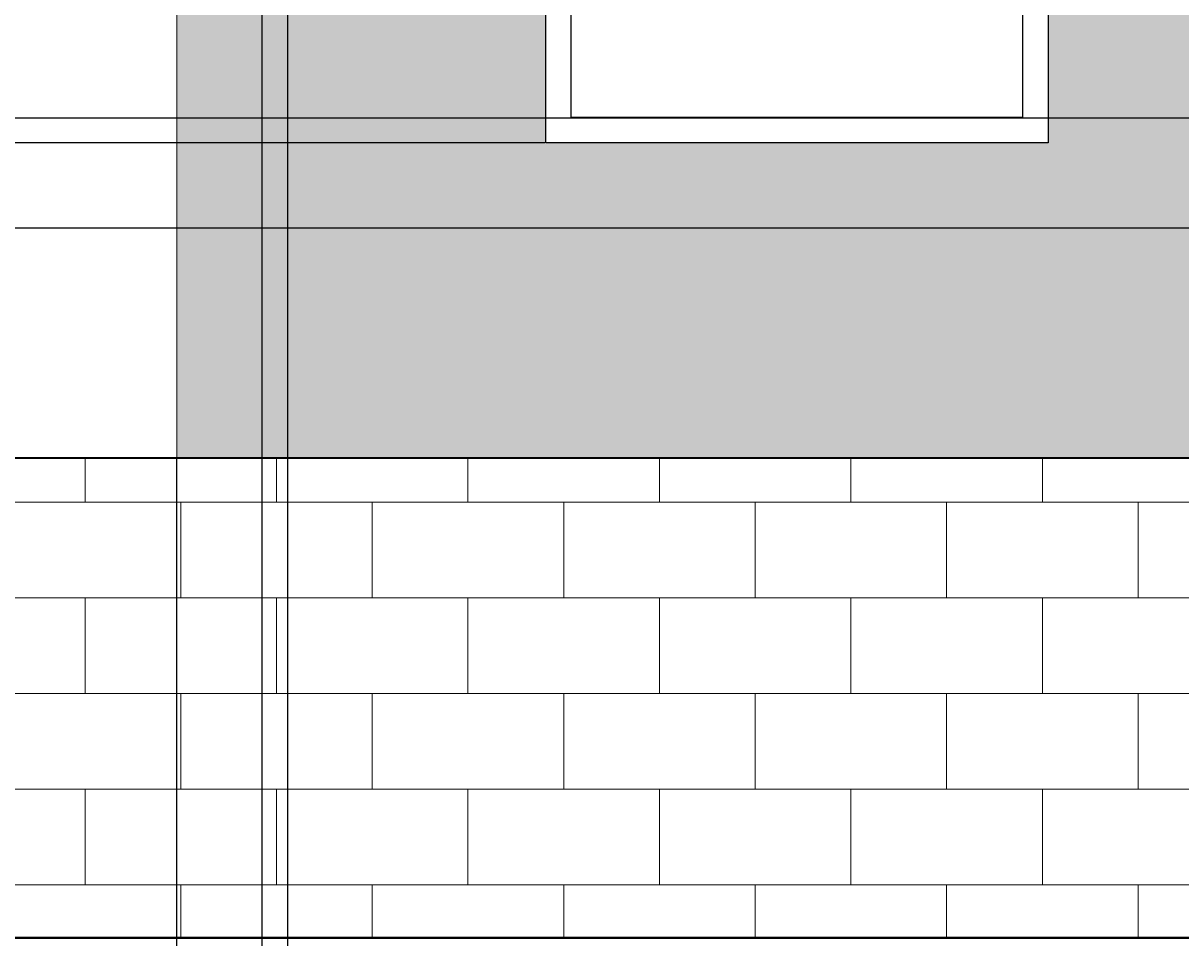
# Model space of a CAD drawing. Units: inches. Extents: x -13 to 809, y 112 to 656.
# Tile 23 of 55: x 430 to 521, y 251 to 323. Entities that reach past the tile are written whole.
import ezdxf

# ---------------------------------------------------------------- set-up
doc = ezdxf.new("R2010")
doc.units = ezdxf.units.IN
doc.header["$MEASUREMENT"] = 0
for name, color, linetype, lineweight in [('A-ANNO-DIMS', 2, 'Continuous', 18), ('A-ELEV', 7, 'Continuous', 35), ('A-ELEV-PATT', 8, 'Continuous', 13), ('A-GLAZ', 4, 'Continuous', 25)]:
    doc.layers.add(name, color=color, linetype=linetype, lineweight=lineweight)
doc.styles.get("Standard").update_dxf_attribs({"font": 'arial.ttf'})
doc.dimstyles.get("Standard").update_dxf_attribs({"dimtxt": 0.625, "dimasz": 0.18, "dimexe": 0.18, "dimexo": 0.0625, "dimgap": 0.09, "dimtad": 0, "dimtih": 1, "dimtoh": 1, "dimdec": 4, "dimzin": 0, "dimdsep": 46, "dimlunit": 4, "dimtxsty": 'Standard', "dimcen": 0.09, "dimadec": 0, "dimazin": 0, "dimtfac": 1, "dimtdec": 4, "dimtofl": 0, "dimtmove": 0, "dimatfit": 3, "dimfxl": 1, "dimtolj": 1, "dimtzin": 0, "dimarcsym": 0})

# ---------------------------------------------------------------- blocks, each defined once
blk = doc.blocks.new('WIN-FIXED-400')
for points in [[(0, 27.268), (39.362, 27.268), (39.362, 0), (0, 0)], [(2, 25.268), (37.362, 25.268), (37.362, 2), (2, 2)]]:
    blk.add_lwpolyline(points, close=True)
blk = doc.blocks.new('*D40')
at = {"layer": 'A-ANNO-DIMS', "color": 0, "lineweight": -2, "transparency": 16777216}
for p, q in [((471.037, 313.167), (-12.099, 313.167)), ((-11.919, 312.987), (-11.919, 301.218)), ((-11.919, 288.631), (-11.919, 300.4)), ((341.345, 288.451), (-12.099, 288.451))]:
    blk.add_line(p, q, dxfattribs=at)
at = {"layer": 'A-ANNO-DIMS', "color": 0, "transparency": 16777216}
for points in [[(-11.949, 312.987), (-11.889, 312.987), (-11.919, 313.167)], [(-11.949, 288.631), (-11.889, 288.631), (-11.919, 288.451)]]:
    blk.add_solid(points, dxfattribs=at)
at = {"layer": 'Defpoints', "color": 0, "transparency": 16777216}
for p in [(471.1, 313.167), (-11.919, 288.451), (341.407, 288.451)]:
    blk.add_point(p, dxfattribs=at)
at = {"layer": 'A-ANNO-DIMS', "color": 0, "transparency": 16777216, "insert": (-11.919, 300.809), "char_height": 0.625, "attachment_point": 5}
blk.add_mtext('\\A1;24.716', dxfattribs=at)
blk = doc.blocks.new('*D41')
at = {"layer": 'A-ANNO-DIMS', "color": 0, "lineweight": -2, "transparency": 16777216}
for p, q in [((471.037, 357.98), (-12.099, 357.98)), ((-11.919, 357.8), (-11.919, 335.983)), ((-11.919, 313.347), (-11.919, 335.164)), ((471.037, 313.167), (-12.099, 313.167))]:
    blk.add_line(p, q, dxfattribs=at)
at = {"layer": 'A-ANNO-DIMS', "color": 0, "transparency": 16777216}
for points in [[(-11.949, 357.8), (-11.889, 357.8), (-11.919, 357.98)], [(-11.949, 313.347), (-11.889, 313.347), (-11.919, 313.167)]]:
    blk.add_solid(points, dxfattribs=at)
at = {"layer": 'Defpoints', "color": 0, "transparency": 16777216}
for p in [(-11.919, 357.98), (471.1, 357.98), (471.1, 313.167)]:
    blk.add_point(p, dxfattribs=at)
at = {"layer": 'A-ANNO-DIMS', "color": 0, "transparency": 16777216, "insert": (-11.919, 335.574), "char_height": 0.625, "attachment_point": 5}
blk.add_mtext('\\A1;44.81', dxfattribs=at)
blk = doc.blocks.new('*D51')
at = {"layer": 'A-ANNO-DIMS', "color": 0, "lineweight": -2, "transparency": 16777216}
for p, q in [((341.407, 288.388), (341.407, 112.34)), ((442.184, 288.388), (442.184, 112.34)), ((341.587, 112.52), (390.437, 112.52)), ((442.004, 112.52), (393.154, 112.52))]:
    blk.add_line(p, q, dxfattribs=at)
at = {"layer": 'A-ANNO-DIMS', "color": 0, "transparency": 16777216}
for points in [[(341.587, 112.55), (341.587, 112.49), (341.407, 112.52)], [(442.004, 112.55), (442.004, 112.49), (442.184, 112.52)]]:
    blk.add_solid(points, dxfattribs=at)
at = {"layer": 'Defpoints', "color": 0, "transparency": 16777216}
for p in [(341.407, 288.451), (442.184, 288.451), (442.184, 112.52)]:
    blk.add_point(p, dxfattribs=at)
at = {"layer": 'A-ANNO-DIMS', "color": 0, "transparency": 16777216, "insert": (391.796, 112.52), "char_height": 0.625, "attachment_point": 5}
blk.add_mtext('\\A1;100.78', dxfattribs=at)
blk = doc.blocks.new('*D52')
at = {"layer": 'A-ANNO-DIMS', "color": 0, "lineweight": -2, "transparency": 16777216}
for p, q in [((442.184, 288.388), (442.184, 112.34)), ((542.962, 288.388), (542.962, 112.34)), ((442.364, 112.52), (491.215, 112.52)), ((542.782, 112.52), (493.932, 112.52))]:
    blk.add_line(p, q, dxfattribs=at)
at = {"layer": 'A-ANNO-DIMS', "color": 0, "transparency": 16777216}
for points in [[(442.364, 112.55), (442.364, 112.49), (442.184, 112.52)], [(542.782, 112.55), (542.782, 112.49), (542.962, 112.52)]]:
    blk.add_solid(points, dxfattribs=at)
at = {"layer": 'Defpoints', "color": 0, "transparency": 16777216}
for p in [(442.184, 288.451), (542.962, 288.451), (542.962, 112.52)]:
    blk.add_point(p, dxfattribs=at)
at = {"layer": 'A-ANNO-DIMS', "color": 0, "transparency": 16777216, "insert": (492.573, 112.52), "char_height": 0.625, "attachment_point": 5}
blk.add_mtext('\\A1;100.78', dxfattribs=at)
blk = doc.blocks.new('*D106')
at = {"layer": 'A-ANNO-DIMS', "color": 0, "lineweight": -2, "transparency": 16777216}
for p, q in [((319.57, 315.144), (807.769, 315.144)), ((807.589, 314.964), (807.589, 311.241)), ((807.589, 306.7), (807.589, 310.423)), ((337.57, 306.52), (807.769, 306.52))]:
    blk.add_line(p, q, dxfattribs=at)
at = {"layer": 'A-ANNO-DIMS', "color": 0, "transparency": 16777216}
for points in [[(807.559, 314.964), (807.619, 314.964), (807.589, 315.144)], [(807.559, 306.7), (807.619, 306.7), (807.589, 306.52)]]:
    blk.add_solid(points, dxfattribs=at)
at = {"layer": 'Defpoints', "color": 0, "transparency": 16777216}
for p in [(319.507, 315.144), (807.589, 315.144), (337.507, 306.52)]:
    blk.add_point(p, dxfattribs=at)
at = {"layer": 'A-ANNO-DIMS', "color": 0, "transparency": 16777216, "insert": (807.589, 310.832), "char_height": 0.625, "attachment_point": 5}
blk.add_mtext('\\A1;8.624', dxfattribs=at)
blk = doc.blocks.new('*D133')
at = {"layer": 'A-ANNO-DIMS', "color": 0, "lineweight": -2, "transparency": 16777216}
for p, q in [((448.701738, 655.782835), (448.521738, 655.782835)), ((448.881738, 207.535185), (448.881738, 655.962835)), ((450.881738, 207.527657), (450.881738, 655.962835)), ((451.061738, 655.782835), (451.241738, 655.782835))]:
    blk.add_line(p, q, dxfattribs=at)
at = {"layer": 'A-ANNO-DIMS', "color": 0, "transparency": 16777216}
for points in [[(448.701738, 655.812835), (448.701738, 655.752835), (448.881738, 655.782835)], [(451.061738, 655.812835), (451.061738, 655.752835), (450.881738, 655.782835)]]:
    blk.add_solid(points, dxfattribs=at)
at = {"layer": 'Defpoints', "color": 0, "transparency": 16777216}
for p in [(450.881738, 655.782835), (448.881738, 207.472685), (450.881738, 207.465157)]:
    blk.add_point(p, dxfattribs=at)
at = {"layer": 'A-ANNO-DIMS', "color": 0, "transparency": 16777216, "insert": (449.881738, 655.782835), "char_height": 0.625, "attachment_point": 5}
blk.add_mtext('\\A1;2.00', dxfattribs=at)

msp = doc.modelspace()

# ---------------------------------------------------------------- hatches: boundary and pattern name
at = {"layer": 'A-ELEV-PATT'}
h = msp.add_hatch(dxfattribs=at)
h.set_pattern_fill('BRICK', color=256, scale=30)
h.paths.add_polyline_path([(591.008, 558.5199), (341.4072, 558.5199), (341.4072, 524.281), (542.9617, 524.281), (542.9617, 288.4508), (341.4072, 288.4508), (341.4072, 250.8429), (591.008, 250.8429)])
h = msp.add_hatch(dxfattribs=at)
h.set_pattern_fill('CROSS', color=256, scale=9.7)
h.paths.add_polyline_path([(542.9617, 524.281), (442.1845, 524.281), (442.1845, 288.4508), (542.9617, 288.4508)])
h.paths.add_polyline_path([(471.0998, 470.8765), (471.0998, 498.1452), (510.462, 498.1452), (510.462, 470.8765)], flags=16)
h.paths.add_polyline_path([(473.0998, 472.8765), (473.0998, 496.1452), (508.462, 496.1452), (508.462, 472.8765)], flags=0)
h.paths.add_polyline_path([(471.0998, 442.128), (510.462, 442.128), (510.462, 414.8594), (471.0998, 414.8594)], flags=16)
h.paths.add_polyline_path([(473.0998, 440.128), (508.462, 440.128), (508.462, 416.8594), (473.0998, 416.8594)], flags=0)
h.paths.add_polyline_path([(471.0998, 385.2491), (510.462, 385.2491), (510.462, 357.9804), (471.0998, 357.9804)], flags=16)
h.paths.add_polyline_path([(473.0998, 383.2491), (508.462, 383.2491), (508.462, 359.9804), (473.0998, 359.9804)], flags=0)
h.paths.add_polyline_path([(471.0998, 340.4353), (510.462, 340.4353), (510.462, 313.1667), (471.0998, 313.1667)], flags=16)
h.paths.add_polyline_path([(473.0998, 338.4353), (508.462, 338.4353), (508.462, 315.1667), (473.0998, 315.1667)], flags=0)

# ---------------------------------------------------------------- linework, layer by layer
at = {"layer": 'A-ELEV'}
msp.add_line((341.4072, 250.8429), (591.008, 250.8429), dxfattribs=at)
for points in [[(341.4072, 558.5199), (591.008, 558.5199), (591.008, 250.8429), (341.4072, 250.8429)], [(341.4072, 524.281), (542.9617, 524.281), (542.9617, 288.4508), (341.4072, 288.4508)]]:
    msp.add_lwpolyline(points, close=True, dxfattribs=at)
at = {"layer": 'A-ELEV-PATT'}
msp.add_line((442.1845, 524.281), (442.1845, 288.4508), dxfattribs=at)

# ---------------------------------------------------------------- block references
at = {"layer": 'A-GLAZ'}
msp.add_blockref('WIN-FIXED-400', (471.1, 313.1672), dxfattribs=at)

# ---------------------------------------------------------------- dimensions: what is measured, and where the dimension line sits
at = {"layer": 'A-ANNO-DIMS'}
for base, p1, p2, picture, middle in [((450.8817, 655.7828), (448.8817, 207.4727), (450.8817, 207.4652), '*D133', (449.8817, 655.7828)), ((442.1845, 112.5199), (341.4072, 288.4508), (442.1845, 288.4508), '*D51', (391.7958, 112.5199)), ((542.9617, 112.5199), (442.1845, 288.4508), (542.9617, 288.4508), '*D52', (492.5731, 112.5199))]:
    dim = msp.add_linear_dim(base=base, p1=p1, p2=p2, dimstyle='Standard', override={"dimdec": 2, "dimlfac": 1, "dimrnd": 0, "dimzin": 0, "dimdsep": 46, "dimlunit": 2}, dxfattribs=at)
    dim.commit()
    dim.dimension.update_dxf_attribs({"geometry": picture, "text_midpoint": middle})
for base, p1, p2, override, picture, middle in [((-11.9191, 357.9804), (471.0998, 313.1667), (471.0998, 357.9804), {"dimdec": 2, "dimlfac": 1, "dimrnd": 0, "dimzin": 0, "dimdsep": 46, "dimlunit": 2}, '*D41', (-11.9191, 335.5735)), ((807.5888, 315.1435), (337.5074, 306.5199), (319.5074, 315.1435), {"dimdec": 3, "dimlfac": 1, "dimrnd": 0, "dimzin": 0, "dimdsep": 46, "dimlunit": 2}, '*D106', (807.5888, 310.8317)), ((-11.9191, 288.4508), (471.0998, 313.1667), (341.4072, 288.4508), {"dimdec": 3, "dimlfac": 1, "dimrnd": 0, "dimzin": 0, "dimdsep": 46, "dimlunit": 2}, '*D40', (-11.9191, 300.8087))]:
    dim = msp.add_linear_dim(base=base, p1=p1, p2=p2, angle=90, dimstyle='Standard', override=override, dxfattribs=at)
    dim.commit()
    dim.dimension.update_dxf_attribs({"geometry": picture, "text_midpoint": middle})

doc.saveas('drawing.dxf')
